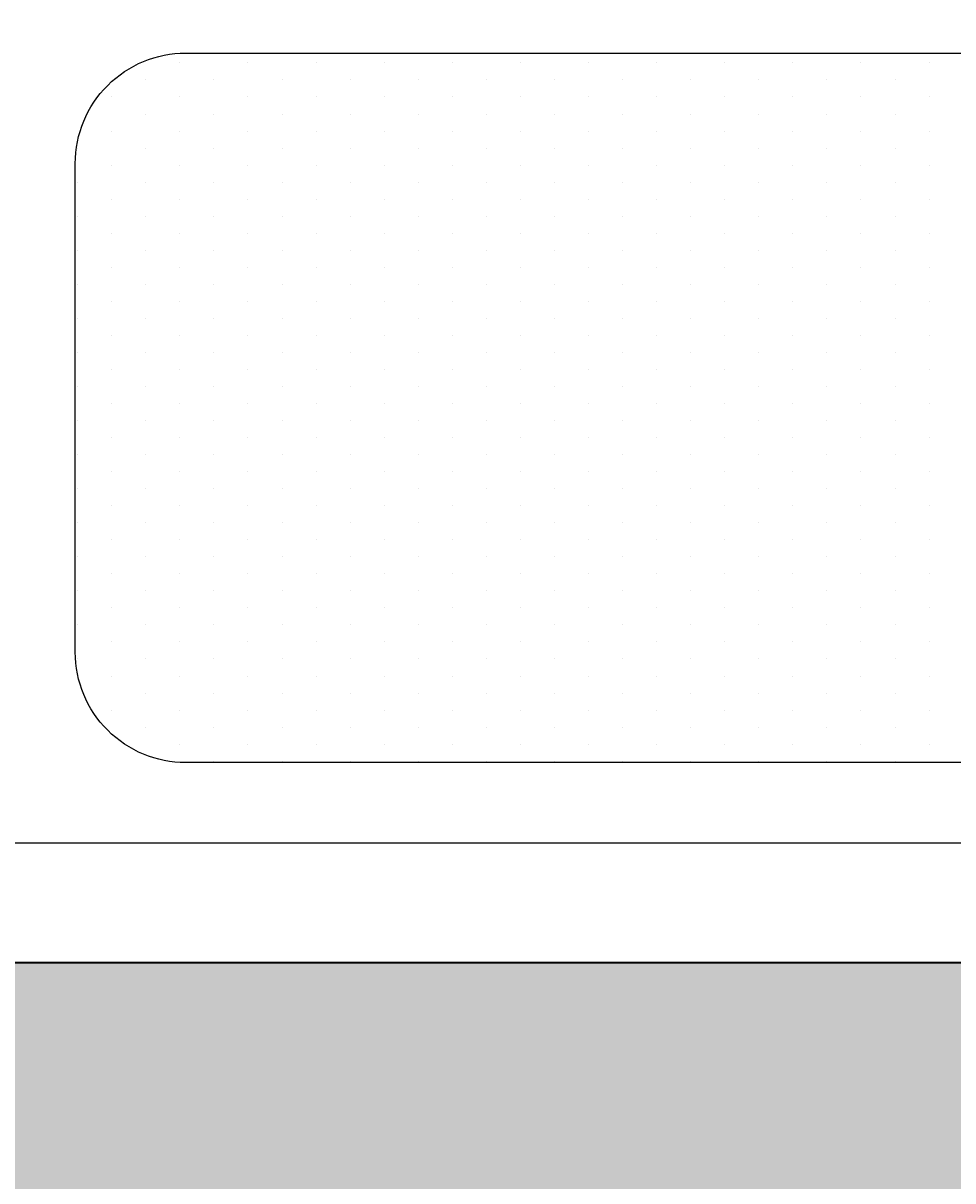
# Model space of a CAD drawing. Units: millimetres. Extents: x 2817 to 5038, y 1110 to 3565.
# Tile 13 of 21: x 2898 to 2917, y 1505 to 1528. Entities that reach past the tile are written whole.
import ezdxf

# ---------------------------------------------------------------- set-up
doc = ezdxf.new("R2010")
doc.units = ezdxf.units.MM
for name, color, linetype, lineweight in [('A-ANNO-DIMS', 2, 'Continuous', 18), ('A-WALL', 7, 'Continuous', 35), ('FURNITURE', 219, 'Continuous', 18)]:
    doc.layers.add(name, color=color, linetype=linetype, lineweight=lineweight)
doc.layers.add('A-WALL-PATT', color=51, linetype='Continuous', lineweight=13, true_color=0xf7f281)
doc.layers.add('BLOCK', color=6, linetype='Continuous')
doc.styles.get("Standard").update_dxf_attribs({"font": 'arial.ttf'})
doc.dimstyles.get("Standard").update_dxf_attribs({"dimtxt": 0.18, "dimasz": 0.18, "dimexe": 0.18, "dimexo": 0.0625, "dimgap": 0.09, "dimtad": 0, "dimtih": 1, "dimtoh": 1, "dimdec": 4, "dimzin": 0, "dimdsep": 46, "dimtxsty": 'Standard', "dimcen": 0.09, "dimadec": 0, "dimazin": 0, "dimtfac": 1, "dimtdec": 4, "dimtofl": 0, "dimtmove": 0, "dimatfit": 3, "dimfxl": 1, "dimtolj": 1, "dimtzin": 0, "dimarcsym": 0})

# ---------------------------------------------------------------- blocks, each defined once
blk = doc.blocks.new('*X9')
at = {"color": 0}
for p, q in [((268.3125, 457.03125), (268.3125, 457.03125)), ((268.6875, 457.03125), (268.6875, 457.03125)), ((269.0625, 457.03125), (269.0625, 457.03125)), ((269.4375, 457.03125), (269.4375, 457.03125)), ((269.8125, 457.03125), (269.8125, 457.03125)), ((270.1875, 457.03125), (270.1875, 457.03125)), ((270.5625, 457.03125), (270.5625, 457.03125)), ((270.9375, 457.03125), (270.9375, 457.03125)), ((271.3125, 457.03125), (271.3125, 457.03125)), ((271.6875, 457.03125), (271.6875, 457.03125)), ((272.0625, 457.03125), (272.0625, 457.03125)), ((268.125, 456.9375), (268.125, 456.9375)), ((268.5, 456.9375), (268.5, 456.9375)), ((268.875, 456.9375), (268.875, 456.9375)), ((269.25, 456.9375), (269.25, 456.9375)), ((269.625, 456.9375), (269.625, 456.9375)), ((270, 456.9375), (270, 456.9375)), ((270.375, 456.9375), (270.375, 456.9375)), ((270.75, 456.9375), (270.75, 456.9375)), ((271.125, 456.9375), (271.125, 456.9375)), ((271.5, 456.9375), (271.5, 456.9375)), ((271.875, 456.9375), (271.875, 456.9375)), ((272.25, 456.9375), (272.25, 456.9375)), ((268.3125, 456.84375), (268.3125, 456.84375)), ((268.6875, 456.84375), (268.6875, 456.84375)), ((269.0625, 456.84375), (269.0625, 456.84375)), ((269.4375, 456.84375), (269.4375, 456.84375)), ((269.8125, 456.84375), (269.8125, 456.84375)), ((270.1875, 456.84375), (270.1875, 456.84375)), ((270.5625, 456.84375), (270.5625, 456.84375)), ((270.9375, 456.84375), (270.9375, 456.84375)), ((271.3125, 456.84375), (271.3125, 456.84375)), ((271.6875, 456.84375), (271.6875, 456.84375)), ((272.0625, 456.84375), (272.0625, 456.84375)), ((272.4375, 456.84375), (272.4375, 456.84375)), ((268.125, 456.75), (268.125, 456.75)), ((268.5, 456.75), (268.5, 456.75)), ((268.875, 456.75), (268.875, 456.75)), ((269.25, 456.75), (269.25, 456.75)), ((269.625, 456.75), (269.625, 456.75)), ((270, 456.75), (270, 456.75)), ((270.375, 456.75), (270.375, 456.75)), ((270.75, 456.75), (270.75, 456.75)), ((271.125, 456.75), (271.125, 456.75)), ((271.5, 456.75), (271.5, 456.75)), ((271.875, 456.75), (271.875, 456.75)), ((272.25, 456.75), (272.25, 456.75)), ((272.625, 456.75), (272.625, 456.75)), ((268.3125, 456.65625), (268.3125, 456.65625)), ((268.6875, 456.65625), (268.6875, 456.65625)), ((269.0625, 456.65625), (269.0625, 456.65625)), ((269.4375, 456.65625), (269.4375, 456.65625)), ((269.8125, 456.65625), (269.8125, 456.65625)), ((270.1875, 456.65625), (270.1875, 456.65625)), ((270.5625, 456.65625), (270.5625, 456.65625)), ((270.9375, 456.65625), (270.9375, 456.65625)), ((271.3125, 456.65625), (271.3125, 456.65625)), ((271.6875, 456.65625), (271.6875, 456.65625)), ((272.0625, 456.65625), (272.0625, 456.65625)), ((272.4375, 456.65625), (272.4375, 456.65625)), ((268.125, 456.5625), (268.125, 456.5625)), ((268.5, 456.5625), (268.5, 456.5625)), ((268.875, 456.5625), (268.875, 456.5625)), ((269.25, 456.5625), (269.25, 456.5625)), ((269.625, 456.5625), (269.625, 456.5625)), ((270, 456.5625), (270, 456.5625)), ((270.375, 456.5625), (270.375, 456.5625)), ((270.75, 456.5625), (270.75, 456.5625)), ((271.125, 456.5625), (271.125, 456.5625)), ((271.5, 456.5625), (271.5, 456.5625)), ((271.875, 456.5625), (271.875, 456.5625)), ((272.25, 456.5625), (272.25, 456.5625)), ((272.625, 456.5625), (272.625, 456.5625)), ((268.3125, 456.46875), (268.3125, 456.46875)), ((268.6875, 456.46875), (268.6875, 456.46875)), ((269.0625, 456.46875), (269.0625, 456.46875)), ((269.4375, 456.46875), (269.4375, 456.46875)), ((269.8125, 456.46875), (269.8125, 456.46875)), ((270.1875, 456.46875), (270.1875, 456.46875)), ((270.5625, 456.46875), (270.5625, 456.46875)), ((270.9375, 456.46875), (270.9375, 456.46875)), ((271.3125, 456.46875), (271.3125, 456.46875)), ((271.6875, 456.46875), (271.6875, 456.46875)), ((272.0625, 456.46875), (272.0625, 456.46875)), ((272.4375, 456.46875), (272.4375, 456.46875)), ((272.8125, 456.46875), (272.8125, 456.46875)), ((268.125, 456.375), (268.125, 456.375)), ((268.5, 456.375), (268.5, 456.375)), ((268.875, 456.375), (268.875, 456.375)), ((269.25, 456.375), (269.25, 456.375)), ((269.625, 456.375), (269.625, 456.375)), ((270, 456.375), (270, 456.375)), ((270.375, 456.375), (270.375, 456.375)), ((270.75, 456.375), (270.75, 456.375)), ((271.125, 456.375), (271.125, 456.375)), ((271.5, 456.375), (271.5, 456.375)), ((271.875, 456.375), (271.875, 456.375)), ((272.25, 456.375), (272.25, 456.375)), ((272.625, 456.375), (272.625, 456.375)), ((268.3125, 456.28125), (268.3125, 456.28125)), ((268.6875, 456.28125), (268.6875, 456.28125)), ((269.0625, 456.28125), (269.0625, 456.28125)), ((269.4375, 456.28125), (269.4375, 456.28125)), ((269.8125, 456.28125), (269.8125, 456.28125)), ((270.1875, 456.28125), (270.1875, 456.28125)), ((270.5625, 456.28125), (270.5625, 456.28125)), ((270.9375, 456.28125), (270.9375, 456.28125)), ((271.3125, 456.28125), (271.3125, 456.28125)), ((271.6875, 456.28125), (271.6875, 456.28125)), ((272.0625, 456.28125), (272.0625, 456.28125)), ((272.4375, 456.28125), (272.4375, 456.28125)), ((272.8125, 456.28125), (272.8125, 456.28125)), ((268.125, 456.1875), (268.125, 456.1875)), ((268.5, 456.1875), (268.5, 456.1875)), ((268.875, 456.1875), (268.875, 456.1875)), ((269.25, 456.1875), (269.25, 456.1875)), ((269.625, 456.1875), (269.625, 456.1875)), ((270, 456.1875), (270, 456.1875)), ((270.375, 456.1875), (270.375, 456.1875)), ((270.75, 456.1875), (270.75, 456.1875)), ((271.125, 456.1875), (271.125, 456.1875)), ((271.5, 456.1875), (271.5, 456.1875)), ((271.875, 456.1875), (271.875, 456.1875)), ((272.25, 456.1875), (272.25, 456.1875)), ((272.625, 456.1875), (272.625, 456.1875)), ((268.3125, 456.09375), (268.3125, 456.09375)), ((268.6875, 456.09375), (268.6875, 456.09375)), ((269.0625, 456.09375), (269.0625, 456.09375)), ((269.4375, 456.09375), (269.4375, 456.09375)), ((269.8125, 456.09375), (269.8125, 456.09375)), ((270.1875, 456.09375), (270.1875, 456.09375)), ((270.5625, 456.09375), (270.5625, 456.09375)), ((270.9375, 456.09375), (270.9375, 456.09375)), ((271.3125, 456.09375), (271.3125, 456.09375)), ((271.6875, 456.09375), (271.6875, 456.09375)), ((272.0625, 456.09375), (272.0625, 456.09375)), ((272.4375, 456.09375), (272.4375, 456.09375)), ((272.8125, 456.09375), (272.8125, 456.09375)), ((268.125, 456), (268.125, 456)), ((268.5, 456), (268.5, 456)), ((268.875, 456), (268.875, 456)), ((269.25, 456), (269.25, 456)), ((269.625, 456), (269.625, 456)), ((270, 456), (270, 456)), ((270.375, 456), (270.375, 456)), ((270.75, 456), (270.75, 456)), ((271.125, 456), (271.125, 456)), ((271.5, 456), (271.5, 456)), ((271.875, 456), (271.875, 456)), ((272.25, 456), (272.25, 456)), ((272.625, 456), (272.625, 456)), ((268.3125, 455.90625), (268.3125, 455.90625)), ((268.6875, 455.90625), (268.6875, 455.90625)), ((269.0625, 455.90625), (269.0625, 455.90625)), ((269.4375, 455.90625), (269.4375, 455.90625)), ((269.8125, 455.90625), (269.8125, 455.90625)), ((270.1875, 455.90625), (270.1875, 455.90625)), ((270.5625, 455.90625), (270.5625, 455.90625)), ((270.9375, 455.90625), (270.9375, 455.90625)), ((271.3125, 455.90625), (271.3125, 455.90625)), ((271.6875, 455.90625), (271.6875, 455.90625)), ((272.0625, 455.90625), (272.0625, 455.90625)), ((272.4375, 455.90625), (272.4375, 455.90625)), ((272.8125, 455.90625), (272.8125, 455.90625)), ((268.125, 455.8125), (268.125, 455.8125)), ((268.5, 455.8125), (268.5, 455.8125)), ((268.875, 455.8125), (268.875, 455.8125)), ((269.25, 455.8125), (269.25, 455.8125)), ((269.625, 455.8125), (269.625, 455.8125)), ((270, 455.8125), (270, 455.8125)), ((270.375, 455.8125), (270.375, 455.8125)), ((270.75, 455.8125), (270.75, 455.8125)), ((271.125, 455.8125), (271.125, 455.8125)), ((271.5, 455.8125), (271.5, 455.8125)), ((271.875, 455.8125), (271.875, 455.8125)), ((272.25, 455.8125), (272.25, 455.8125)), ((272.625, 455.8125), (272.625, 455.8125)), ((268.3125, 455.71875), (268.3125, 455.71875)), ((268.6875, 455.71875), (268.6875, 455.71875)), ((269.0625, 455.71875), (269.0625, 455.71875)), ((269.4375, 455.71875), (269.4375, 455.71875)), ((269.8125, 455.71875), (269.8125, 455.71875)), ((270.1875, 455.71875), (270.1875, 455.71875)), ((270.5625, 455.71875), (270.5625, 455.71875)), ((270.9375, 455.71875), (270.9375, 455.71875)), ((271.3125, 455.71875), (271.3125, 455.71875)), ((271.6875, 455.71875), (271.6875, 455.71875)), ((272.0625, 455.71875), (272.0625, 455.71875)), ((272.4375, 455.71875), (272.4375, 455.71875)), ((272.8125, 455.71875), (272.8125, 455.71875)), ((268.125, 455.625), (268.125, 455.625)), ((268.5, 455.625), (268.5, 455.625)), ((268.875, 455.625), (268.875, 455.625)), ((269.25, 455.625), (269.25, 455.625)), ((269.625, 455.625), (269.625, 455.625)), ((270, 455.625), (270, 455.625)), ((270.375, 455.625), (270.375, 455.625)), ((270.75, 455.625), (270.75, 455.625)), ((271.125, 455.625), (271.125, 455.625)), ((271.5, 455.625), (271.5, 455.625)), ((271.875, 455.625), (271.875, 455.625)), ((272.25, 455.625), (272.25, 455.625)), ((272.625, 455.625), (272.625, 455.625)), ((268.3125, 455.53125), (268.3125, 455.53125)), ((268.6875, 455.53125), (268.6875, 455.53125)), ((269.0625, 455.53125), (269.0625, 455.53125)), ((269.4375, 455.53125), (269.4375, 455.53125)), ((269.8125, 455.53125), (269.8125, 455.53125)), ((270.1875, 455.53125), (270.1875, 455.53125)), ((270.5625, 455.53125), (270.5625, 455.53125)), ((270.9375, 455.53125), (270.9375, 455.53125)), ((271.3125, 455.53125), (271.3125, 455.53125)), ((271.6875, 455.53125), (271.6875, 455.53125)), ((272.0625, 455.53125), (272.0625, 455.53125)), ((272.4375, 455.53125), (272.4375, 455.53125)), ((272.8125, 455.53125), (272.8125, 455.53125)), ((268.125, 455.4375), (268.125, 455.4375)), ((268.5, 455.4375), (268.5, 455.4375)), ((268.875, 455.4375), (268.875, 455.4375)), ((269.25, 455.4375), (269.25, 455.4375)), ((269.625, 455.4375), (269.625, 455.4375)), ((270, 455.4375), (270, 455.4375)), ((270.375, 455.4375), (270.375, 455.4375)), ((270.75, 455.4375), (270.75, 455.4375)), ((271.125, 455.4375), (271.125, 455.4375)), ((271.5, 455.4375), (271.5, 455.4375)), ((271.875, 455.4375), (271.875, 455.4375)), ((272.25, 455.4375), (272.25, 455.4375)), ((272.625, 455.4375), (272.625, 455.4375)), ((268.3125, 455.34375), (268.3125, 455.34375)), ((268.6875, 455.34375), (268.6875, 455.34375)), ((269.0625, 455.34375), (269.0625, 455.34375)), ((269.4375, 455.34375), (269.4375, 455.34375)), ((269.8125, 455.34375), (269.8125, 455.34375)), ((270.1875, 455.34375), (270.1875, 455.34375)), ((270.5625, 455.34375), (270.5625, 455.34375)), ((270.9375, 455.34375), (270.9375, 455.34375)), ((271.3125, 455.34375), (271.3125, 455.34375)), ((271.6875, 455.34375), (271.6875, 455.34375)), ((272.0625, 455.34375), (272.0625, 455.34375)), ((272.4375, 455.34375), (272.4375, 455.34375)), ((272.8125, 455.34375), (272.8125, 455.34375)), ((268.125, 455.25), (268.125, 455.25)), ((268.5, 455.25), (268.5, 455.25)), ((268.875, 455.25), (268.875, 455.25)), ((269.25, 455.25), (269.25, 455.25)), ((269.625, 455.25), (269.625, 455.25)), ((270, 455.25), (270, 455.25)), ((270.375, 455.25), (270.375, 455.25)), ((270.75, 455.25), (270.75, 455.25)), ((271.125, 455.25), (271.125, 455.25)), ((271.5, 455.25), (271.5, 455.25)), ((271.875, 455.25), (271.875, 455.25)), ((272.25, 455.25), (272.25, 455.25)), ((272.625, 455.25), (272.625, 455.25)), ((268.3125, 455.15625), (268.3125, 455.15625)), ((268.6875, 455.15625), (268.6875, 455.15625)), ((269.0625, 455.15625), (269.0625, 455.15625)), ((269.4375, 455.15625), (269.4375, 455.15625)), ((269.8125, 455.15625), (269.8125, 455.15625)), ((270.1875, 455.15625), (270.1875, 455.15625)), ((270.5625, 455.15625), (270.5625, 455.15625)), ((270.9375, 455.15625), (270.9375, 455.15625)), ((271.3125, 455.15625), (271.3125, 455.15625)), ((271.6875, 455.15625), (271.6875, 455.15625)), ((272.0625, 455.15625), (272.0625, 455.15625)), ((272.4375, 455.15625), (272.4375, 455.15625)), ((272.8125, 455.15625), (272.8125, 455.15625)), ((268.125, 455.0625), (268.125, 455.0625)), ((268.5, 455.0625), (268.5, 455.0625)), ((268.875, 455.0625), (268.875, 455.0625)), ((269.25, 455.0625), (269.25, 455.0625)), ((269.625, 455.0625), (269.625, 455.0625)), ((270, 455.0625), (270, 455.0625)), ((270.375, 455.0625), (270.375, 455.0625)), ((270.75, 455.0625), (270.75, 455.0625)), ((271.125, 455.0625), (271.125, 455.0625)), ((271.5, 455.0625), (271.5, 455.0625)), ((271.875, 455.0625), (271.875, 455.0625)), ((272.25, 455.0625), (272.25, 455.0625)), ((272.625, 455.0625), (272.625, 455.0625)), ((268.3125, 454.96875), (268.3125, 454.96875)), ((268.6875, 454.96875), (268.6875, 454.96875)), ((269.0625, 454.96875), (269.0625, 454.96875)), ((269.4375, 454.96875), (269.4375, 454.96875)), ((269.8125, 454.96875), (269.8125, 454.96875)), ((270.1875, 454.96875), (270.1875, 454.96875)), ((270.5625, 454.96875), (270.5625, 454.96875)), ((270.9375, 454.96875), (270.9375, 454.96875)), ((271.3125, 454.96875), (271.3125, 454.96875)), ((271.6875, 454.96875), (271.6875, 454.96875)), ((272.0625, 454.96875), (272.0625, 454.96875)), ((272.4375, 454.96875), (272.4375, 454.96875)), ((272.8125, 454.96875), (272.8125, 454.96875)), ((268.125, 454.875), (268.125, 454.875)), ((268.5, 454.875), (268.5, 454.875)), ((268.875, 454.875), (268.875, 454.875)), ((269.25, 454.875), (269.25, 454.875)), ((269.625, 454.875), (269.625, 454.875)), ((270, 454.875), (270, 454.875)), ((270.375, 454.875), (270.375, 454.875)), ((270.75, 454.875), (270.75, 454.875)), ((271.125, 454.875), (271.125, 454.875)), ((271.5, 454.875), (271.5, 454.875)), ((271.875, 454.875), (271.875, 454.875)), ((272.25, 454.875), (272.25, 454.875)), ((272.625, 454.875), (272.625, 454.875)), ((268.3125, 454.78125), (268.3125, 454.78125)), ((268.6875, 454.78125), (268.6875, 454.78125)), ((269.0625, 454.78125), (269.0625, 454.78125)), ((269.4375, 454.78125), (269.4375, 454.78125)), ((269.8125, 454.78125), (269.8125, 454.78125)), ((270.1875, 454.78125), (270.1875, 454.78125)), ((270.5625, 454.78125), (270.5625, 454.78125)), ((270.9375, 454.78125), (270.9375, 454.78125)), ((271.3125, 454.78125), (271.3125, 454.78125)), ((271.6875, 454.78125), (271.6875, 454.78125)), ((272.0625, 454.78125), (272.0625, 454.78125)), ((272.4375, 454.78125), (272.4375, 454.78125)), ((272.8125, 454.78125), (272.8125, 454.78125)), ((268.125, 454.6875), (268.125, 454.6875)), ((268.5, 454.6875), (268.5, 454.6875)), ((268.875, 454.6875), (268.875, 454.6875)), ((269.25, 454.6875), (269.25, 454.6875)), ((269.625, 454.6875), (269.625, 454.6875)), ((270, 454.6875), (270, 454.6875)), ((270.375, 454.6875), (270.375, 454.6875)), ((270.75, 454.6875), (270.75, 454.6875)), ((271.125, 454.6875), (271.125, 454.6875)), ((271.5, 454.6875), (271.5, 454.6875)), ((271.875, 454.6875), (271.875, 454.6875)), ((272.25, 454.6875), (272.25, 454.6875)), ((272.625, 454.6875), (272.625, 454.6875)), ((268.3125, 454.59375), (268.3125, 454.59375)), ((268.6875, 454.59375), (268.6875, 454.59375)), ((269.0625, 454.59375), (269.0625, 454.59375)), ((269.4375, 454.59375), (269.4375, 454.59375)), ((269.8125, 454.59375), (269.8125, 454.59375)), ((270.1875, 454.59375), (270.1875, 454.59375)), ((270.5625, 454.59375), (270.5625, 454.59375)), ((270.9375, 454.59375), (270.9375, 454.59375)), ((271.3125, 454.59375), (271.3125, 454.59375)), ((271.6875, 454.59375), (271.6875, 454.59375)), ((272.0625, 454.59375), (272.0625, 454.59375)), ((272.4375, 454.59375), (272.4375, 454.59375)), ((272.8125, 454.59375), (272.8125, 454.59375)), ((268.125, 454.5), (268.125, 454.5)), ((268.5, 454.5), (268.5, 454.5)), ((268.875, 454.5), (268.875, 454.5)), ((269.25, 454.5), (269.25, 454.5)), ((269.625, 454.5), (269.625, 454.5)), ((270, 454.5), (270, 454.5)), ((270.375, 454.5), (270.375, 454.5)), ((270.75, 454.5), (270.75, 454.5)), ((271.125, 454.5), (271.125, 454.5)), ((271.5, 454.5), (271.5, 454.5)), ((271.875, 454.5), (271.875, 454.5)), ((272.25, 454.5), (272.25, 454.5)), ((272.625, 454.5), (272.625, 454.5)), ((268.3125, 454.40625), (268.3125, 454.40625)), ((268.6875, 454.40625), (268.6875, 454.40625)), ((269.0625, 454.40625), (269.0625, 454.40625)), ((269.4375, 454.40625), (269.4375, 454.40625)), ((269.8125, 454.40625), (269.8125, 454.40625)), ((270.1875, 454.40625), (270.1875, 454.40625)), ((270.5625, 454.40625), (270.5625, 454.40625)), ((270.9375, 454.40625), (270.9375, 454.40625)), ((271.3125, 454.40625), (271.3125, 454.40625)), ((271.6875, 454.40625), (271.6875, 454.40625)), ((272.0625, 454.40625), (272.0625, 454.40625)), ((272.4375, 454.40625), (272.4375, 454.40625)), ((272.8125, 454.40625), (272.8125, 454.40625)), ((268.125, 454.3125), (268.125, 454.3125)), ((268.5, 454.3125), (268.5, 454.3125)), ((268.875, 454.3125), (268.875, 454.3125)), ((269.25, 454.3125), (269.25, 454.3125)), ((269.625, 454.3125), (269.625, 454.3125)), ((270, 454.3125), (270, 454.3125)), ((270.375, 454.3125), (270.375, 454.3125)), ((270.75, 454.3125), (270.75, 454.3125)), ((271.125, 454.3125), (271.125, 454.3125)), ((271.5, 454.3125), (271.5, 454.3125)), ((271.875, 454.3125), (271.875, 454.3125)), ((272.25, 454.3125), (272.25, 454.3125)), ((272.625, 454.3125), (272.625, 454.3125)), ((268.3125, 454.21875), (268.3125, 454.21875)), ((268.6875, 454.21875), (268.6875, 454.21875)), ((269.0625, 454.21875), (269.0625, 454.21875)), ((269.4375, 454.21875), (269.4375, 454.21875)), ((269.8125, 454.21875), (269.8125, 454.21875)), ((270.1875, 454.21875), (270.1875, 454.21875)), ((270.5625, 454.21875), (270.5625, 454.21875)), ((270.9375, 454.21875), (270.9375, 454.21875)), ((271.3125, 454.21875), (271.3125, 454.21875)), ((271.6875, 454.21875), (271.6875, 454.21875)), ((272.0625, 454.21875), (272.0625, 454.21875)), ((272.4375, 454.21875), (272.4375, 454.21875)), ((272.8125, 454.21875), (272.8125, 454.21875)), ((268.125, 454.125), (268.125, 454.125)), ((268.5, 454.125), (268.5, 454.125)), ((268.875, 454.125), (268.875, 454.125)), ((269.25, 454.125), (269.25, 454.125)), ((269.625, 454.125), (269.625, 454.125)), ((270, 454.125), (270, 454.125)), ((270.375, 454.125), (270.375, 454.125)), ((270.75, 454.125), (270.75, 454.125)), ((271.125, 454.125), (271.125, 454.125)), ((271.5, 454.125), (271.5, 454.125)), ((271.875, 454.125), (271.875, 454.125)), ((272.25, 454.125), (272.25, 454.125)), ((272.625, 454.125), (272.625, 454.125)), ((268.3125, 454.03125), (268.3125, 454.03125)), ((268.6875, 454.03125), (268.6875, 454.03125)), ((269.0625, 454.03125), (269.0625, 454.03125)), ((269.4375, 454.03125), (269.4375, 454.03125)), ((269.8125, 454.03125), (269.8125, 454.03125)), ((270.1875, 454.03125), (270.1875, 454.03125)), ((270.5625, 454.03125), (270.5625, 454.03125)), ((270.9375, 454.03125), (270.9375, 454.03125)), ((271.3125, 454.03125), (271.3125, 454.03125)), ((271.6875, 454.03125), (271.6875, 454.03125)), ((272.0625, 454.03125), (272.0625, 454.03125)), ((272.4375, 454.03125), (272.4375, 454.03125)), ((272.8125, 454.03125), (272.8125, 454.03125)), ((268.125, 453.9375), (268.125, 453.9375)), ((268.5, 453.9375), (268.5, 453.9375)), ((268.875, 453.9375), (268.875, 453.9375)), ((269.25, 453.9375), (269.25, 453.9375)), ((269.625, 453.9375), (269.625, 453.9375)), ((270, 453.9375), (270, 453.9375)), ((270.375, 453.9375), (270.375, 453.9375)), ((270.75, 453.9375), (270.75, 453.9375)), ((271.125, 453.9375), (271.125, 453.9375)), ((271.5, 453.9375), (271.5, 453.9375)), ((271.875, 453.9375), (271.875, 453.9375)), ((272.25, 453.9375), (272.25, 453.9375)), ((272.625, 453.9375), (272.625, 453.9375)), ((268.3125, 453.84375), (268.3125, 453.84375)), ((268.6875, 453.84375), (268.6875, 453.84375)), ((269.0625, 453.84375), (269.0625, 453.84375)), ((269.4375, 453.84375), (269.4375, 453.84375)), ((269.8125, 453.84375), (269.8125, 453.84375)), ((270.1875, 453.84375), (270.1875, 453.84375)), ((270.5625, 453.84375), (270.5625, 453.84375)), ((270.9375, 453.84375), (270.9375, 453.84375)), ((271.3125, 453.84375), (271.3125, 453.84375)), ((271.6875, 453.84375), (271.6875, 453.84375)), ((272.0625, 453.84375), (272.0625, 453.84375)), ((272.4375, 453.84375), (272.4375, 453.84375)), ((272.8125, 453.84375), (272.8125, 453.84375)), ((268.125, 453.75), (268.125, 453.75)), ((268.5, 453.75), (268.5, 453.75)), ((268.875, 453.75), (268.875, 453.75)), ((269.25, 453.75), (269.25, 453.75)), ((269.625, 453.75), (269.625, 453.75)), ((270, 453.75), (270, 453.75)), ((270.375, 453.75), (270.375, 453.75)), ((270.75, 453.75), (270.75, 453.75)), ((271.125, 453.75), (271.125, 453.75)), ((271.5, 453.75), (271.5, 453.75)), ((271.875, 453.75), (271.875, 453.75)), ((272.25, 453.75), (272.25, 453.75)), ((272.625, 453.75), (272.625, 453.75)), ((268.3125, 453.65625), (268.3125, 453.65625)), ((268.6875, 453.65625), (268.6875, 453.65625)), ((269.0625, 453.65625), (269.0625, 453.65625)), ((269.4375, 453.65625), (269.4375, 453.65625)), ((269.8125, 453.65625), (269.8125, 453.65625)), ((270.1875, 453.65625), (270.1875, 453.65625)), ((270.5625, 453.65625), (270.5625, 453.65625)), ((270.9375, 453.65625), (270.9375, 453.65625)), ((271.3125, 453.65625), (271.3125, 453.65625)), ((271.6875, 453.65625), (271.6875, 453.65625)), ((272.0625, 453.65625), (272.0625, 453.65625)), ((272.4375, 453.65625), (272.4375, 453.65625)), ((272.8125, 453.65625), (272.8125, 453.65625)), ((268.125, 453.5625), (268.125, 453.5625)), ((268.5, 453.5625), (268.5, 453.5625)), ((268.875, 453.5625), (268.875, 453.5625)), ((269.25, 453.5625), (269.25, 453.5625)), ((269.625, 453.5625), (269.625, 453.5625)), ((270, 453.5625), (270, 453.5625)), ((270.375, 453.5625), (270.375, 453.5625)), ((270.75, 453.5625), (270.75, 453.5625)), ((271.125, 453.5625), (271.125, 453.5625)), ((271.5, 453.5625), (271.5, 453.5625)), ((271.875, 453.5625), (271.875, 453.5625)), ((272.25, 453.5625), (272.25, 453.5625)), ((272.625, 453.5625), (272.625, 453.5625)), ((268.3125, 453.46875), (268.3125, 453.46875)), ((268.6875, 453.46875), (268.6875, 453.46875)), ((269.0625, 453.46875), (269.0625, 453.46875)), ((269.4375, 453.46875), (269.4375, 453.46875)), ((269.8125, 453.46875), (269.8125, 453.46875)), ((270.1875, 453.46875), (270.1875, 453.46875)), ((270.5625, 453.46875), (270.5625, 453.46875)), ((270.9375, 453.46875), (270.9375, 453.46875)), ((271.3125, 453.46875), (271.3125, 453.46875)), ((271.6875, 453.46875), (271.6875, 453.46875)), ((272.0625, 453.46875), (272.0625, 453.46875)), ((272.4375, 453.46875), (272.4375, 453.46875)), ((268.125, 453.375), (268.125, 453.375)), ((268.5, 453.375), (268.5, 453.375)), ((268.875, 453.375), (268.875, 453.375)), ((269.25, 453.375), (269.25, 453.375)), ((269.625, 453.375), (269.625, 453.375)), ((270, 453.375), (270, 453.375)), ((270.375, 453.375), (270.375, 453.375)), ((270.75, 453.375), (270.75, 453.375)), ((271.125, 453.375), (271.125, 453.375)), ((271.5, 453.375), (271.5, 453.375)), ((271.875, 453.375), (271.875, 453.375)), ((272.25, 453.375), (272.25, 453.375)), ((272.625, 453.375), (272.625, 453.375)), ((268.3125, 453.28125), (268.3125, 453.28125)), ((268.6875, 453.28125), (268.6875, 453.28125)), ((269.0625, 453.28125), (269.0625, 453.28125)), ((269.4375, 453.28125), (269.4375, 453.28125)), ((269.8125, 453.28125), (269.8125, 453.28125)), ((270.1875, 453.28125), (270.1875, 453.28125)), ((270.5625, 453.28125), (270.5625, 453.28125)), ((270.9375, 453.28125), (270.9375, 453.28125)), ((271.3125, 453.28125), (271.3125, 453.28125)), ((271.6875, 453.28125), (271.6875, 453.28125)), ((272.0625, 453.28125), (272.0625, 453.28125)), ((272.4375, 453.28125), (272.4375, 453.28125)), ((268.125, 453.1875), (268.125, 453.1875)), ((268.5, 453.1875), (268.5, 453.1875)), ((268.875, 453.1875), (268.875, 453.1875)), ((269.25, 453.1875), (269.25, 453.1875)), ((269.625, 453.1875), (269.625, 453.1875)), ((270, 453.1875), (270, 453.1875)), ((270.375, 453.1875), (270.375, 453.1875)), ((270.75, 453.1875), (270.75, 453.1875)), ((271.125, 453.1875), (271.125, 453.1875)), ((271.5, 453.1875), (271.5, 453.1875)), ((271.875, 453.1875), (271.875, 453.1875)), ((272.25, 453.1875), (272.25, 453.1875))]:
    blk.add_line(p, q, dxfattribs=at)
blk = doc.blocks.new('A$C52E67D0D')
at = {"layer": 'BLOCK'}
for points in [[(1901, 0), (601, 0, -0.414214), (501, 100), (501, 1700, -0.414214), (601, 1800), (1901, 1800, -0.414214), (2001, 1700), (2001, 100, -0.414214)], [(1171.77, 1365.08), (595.83, 1365.08, -0.414214), (534.98, 1425.93), (534.98, 1694.83, -0.414214), (595.83, 1755.67), (1171.77, 1755.67, -0.414214), (1232.61, 1694.83), (1232.61, 1425.93, -0.414214)]]:
    blk.add_lwpolyline(points, format="xyb", close=True, dxfattribs=at)
blk.add_arc((1888.63, -1664.54), 3015.26, 87.86419, 117.40011, dxfattribs=at)
at = {"layer": 'BLOCK', "xscale": 100, "yscale": 100, "zscale": 100}
blk.add_blockref('*X9', (-26049.96, -43948.24), dxfattribs=at)
blk = doc.blocks.new('*D38')
at = {"layer": 'A-ANNO-DIMS', "color": 0, "lineweight": -2, "transparency": 16777216}
for p, q in [((3110.177, 1573.436), (2817.308, 1573.436)), ((2817.488, 1573.256), (2817.488, 1523.618)), ((2817.488, 1473.616), (2817.488, 1523.254)), ((3105.677, 1473.436), (2817.308, 1473.436))]:
    blk.add_line(p, q, dxfattribs=at)
for points in [[(2817.458, 1573.256), (2817.518, 1573.256), (2817.488, 1573.436)], [(2817.458, 1473.616), (2817.518, 1473.616), (2817.488, 1473.436)]]:
    blk.add_solid(points, dxfattribs=at)
at = {"layer": 'Defpoints', "color": 0, "lineweight": -2, "transparency": 16777216}
for p in [(2817.488, 1573.436), (3110.239, 1573.436), (3105.739, 1473.436)]:
    blk.add_point(p, dxfattribs=at)
at = {"layer": 'A-ANNO-DIMS', "color": 0, "transparency": 16777216, "insert": (2817.488, 1523.436), "char_height": 0.18, "attachment_point": 5}
blk.add_mtext('\\A1;100', dxfattribs=at)

msp = doc.modelspace()

# ---------------------------------------------------------------- hatches: boundary and pattern name
at = {"layer": 'A-WALL-PATT'}
h = msp.add_hatch(color=256, dxfattribs=at)
h.dxf.hatch_style = 1
h.paths.add_polyline_path([(3061.2393, 1549.7835), (3052.2393, 1549.7835), (3052.2393, 1509.4357), (2991.7393, 1509.4357), (2991.7393, 1575.4357), (2982.7393, 1575.4357), (2982.7393, 1509.4357), (2982.7393, 1500.4357), (3052.2393, 1500.4357), (3052.2393, 1498.4661), (3061.2393, 1498.613)])
h.paths.add_polyline_path([(2946.7393, 1505.8357), (2946.7393, 1509.4357), (2850.7393, 1509.4357), (2850.7393, 1520.7609), (2841.7393, 1520.7609), (2841.7393, 1427.2177), (2850.7393, 1427.3646), (2850.7393, 1500.4357), (2922.7393, 1500.4357), (2931.7393, 1500.4357), (2946.7393, 1500.4357)])
h.paths.add_polyline_path([(3061.2393, 1450.613), (3052.2393, 1450.613), (3052.2393, 1431.4357), (3059.4393, 1431.4357), (3061.2393, 1431.4357)])
h.paths.add_polyline_path([(3061.2393, 1211.2899), (3052.2393, 1211.2899), (3052.2393, 1195.4357), (3059.4393, 1195.4357), (3061.2393, 1195.4357)])

# ---------------------------------------------------------------- linework, layer by layer
at = {"layer": 'A-WALL'}
msp.add_line((2850.7393, 1509.4357), (2946.7393, 1509.4357), dxfattribs=at)

# ---------------------------------------------------------------- block references
at = {"layer": 'FURNITURE', "xscale": 0.0367705835331598, "yscale": 0.0367705835331598, "zscale": 0.0367705835331598, "rotation": 180}
msp.add_blockref('A$C52E67D0D', (2944.3285, 1578.0385), dxfattribs=at)

# ---------------------------------------------------------------- dimensions: what is measured, and where the dimension line sits
at = {"layer": 'A-ANNO-DIMS'}
dim = msp.add_linear_dim(base=(2817.4881, 1573.4357), p1=(3105.7393, 1473.4357), p2=(3110.2393, 1573.4357), angle=90, dimstyle='Standard', override={"dimdec": 0, "dimlfac": 1, "dimrnd": 0, "dimzin": 0, "dimdsep": 46, "dimlunit": 2}, dxfattribs=at)
dim.commit()
dim.dimension.update_dxf_attribs({"geometry": '*D38', "text_midpoint": (2817.4881, 1523.4357)})

doc.saveas('drawing.dxf')
